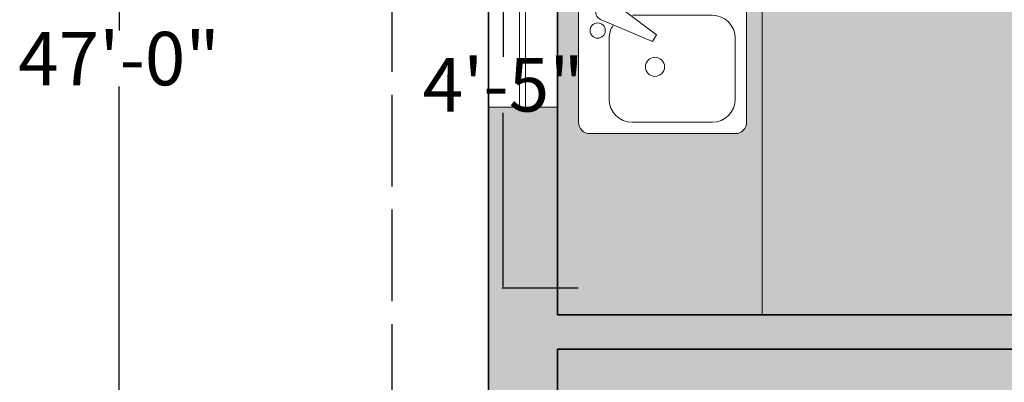
# Model space of a CAD drawing. Units: inches. Extents: x 1316 to 1777, y 813 to 1650.
# Tile 6 of 22: x 1316 to 1445, y 1237 to 1284. Entities that reach past the tile are written whole.
import ezdxf

# ---------------------------------------------------------------- set-up
doc = ezdxf.new("R2010")
doc.units = ezdxf.units.IN
doc.header["$MEASUREMENT"] = 0
doc.linetypes.add('ACAD_ISO02W100', pattern=[15, 12, -3])
for name, color, linetype, lineweight in [('A-ANNO-DIMS', 2, 'Continuous', 18), ('A-FLOR-CASE', 23, 'Continuous', 18), ('A-FLOR-CASE-PATT', 252, 'Continuous', 13), ('A-FLOR-FIXT', 8, 'Continuous', 18), ('A-WALL-PATT', 250, 'Continuous', 13), ('C-PROP', 8, 'ACAD_ISO02W100', 25), ('walls', 250, 'Continuous', 35), ('windows', 141, 'Continuous', 18)]:
    doc.layers.add(name, color=color, linetype=linetype, lineweight=lineweight)
doc.layers.add('A-FLOR-PATT', color=254, linetype='Continuous', lineweight=13, true_color=0xfeeab9)
doc.styles.add('ATT', font='TXT')
doc.styles.get("Standard").update_dxf_attribs({"font": 'arial.ttf'})
doc.dimstyles.get("Standard").update_dxf_attribs({"dimtxt": 7, "dimasz": 0.18, "dimexe": 0.18, "dimexo": 0.0625, "dimgap": 0.09, "dimtad": 0, "dimtih": 1, "dimtoh": 1, "dimzin": 0, "dimdsep": 46, "dimlunit": 3, "dimtxsty": 'Standard', "dimcen": 0.09, "dimadec": 0, "dimazin": 0, "dimtfac": 1, "dimtofl": 0, "dimtmove": 0, "dimatfit": 3, "dimfxl": 1, "dimtolj": 1, "dimtzin": 0, "dimarcsym": 0})

# ---------------------------------------------------------------- blocks, each defined once
blk = doc.blocks.new('15PSNK10')
at = {"color": 0, "linetype": 'ByBlock'}
for p, q in [((20.5, 16.5), (1.5, 16.5)), ((0, 15), (0, -15)), ((7, 15), (17.5, 15)), ((22, -15), (22, 15)), ((4, 4), (4, 12)), ((20.5, 12), (20.5, 4)), ((2.365550999999996, -0.0988979999999984), (2.768423999999995, 0.5988979999999984)), ((10.17820310567643, -3.566986483662404), (4.270020000000002, 0.8709410000000019)), ((17.5, 1), (7, 1)), ((7.038591832997624, -1), (17.5, -1)), ((2.880752999999998, -1.535340000000005), (9.678203105676431, -4.433012483662395)), ((9.678203105676431, -4.433012483662395), (10.17820310567643, -3.566986483662404)), ((4, -12), (4, -4)), ((20.5, -4), (20.5, -12)), ((17.5, -15), (7, -15)), ((1.5, -16.5), (20.5, -16.5))]:
    blk.add_line(p, q, dxfattribs=at)
for centre, radius in [((10, 7.75), 1.25), ((2.5, 3), 1), ((2.5, -3), 1), ((10, -7.75), 1.25)]:
    blk.add_circle(centre, radius, dxfattribs=at)
for centre, radius, start, end in [((1.5, 15), 1.5, 90, 180), ((20.5, 15), 1.5, 0, 90), ((7, 12), 3, 90, 180), ((17.5, 12), 3, 0, 90), ((7, 4), 3, 180, 270), ((17.5, 4), 3, 270, 0), ((3.634449000000003, 0.0988979999999984), 1, 50.537678, 150), ((3.231576000000004, -0.5988979999999984), 1, 150, 249.462322), ((17.5, -4), 3, 0, 90), ((7, -4), 3, 146.6070344853579, 180), ((7, -12), 3, 180, 270), ((17.5, -12), 3, 270, 0), ((1.5, -15), 1.5, 180, 270), ((20.5, -15), 1.5, 270, 0)]:
    blk.add_arc(centre, radius, start, end, dxfattribs=at)
at = {"color": 0, "linetype": 'ByBlock', "style": 'ATT'}
for tag, p, flags in [('ITEM', (0, -26), 3), ('ROOM_NUMBER', (0, -35), 1)]:
    blk.add_attdef(tag, p, '', height=6, dxfattribs=dict(at, flags=flags))
blk = doc.blocks.new('*D23')
at = {"layer": 'A-ANNO-DIMS', "color": 0, "lineweight": -2, "transparency": 16777216}
for p, q in [((1328.466746604303, 1604.172951843256), (1328.865516882555, 1604.172951843256)), ((1328.685516882555, 1603.992951843256), (1328.685516882555, 1282.594977494184)), ((1328.685516882555, 953.868981317008), (1328.685516882555, 1275.26695566608)), ((1328.466746604303, 953.688981317008), (1328.865516882556, 953.688981317008))]:
    blk.add_line(p, q, dxfattribs=at)
at = {"layer": 'A-ANNO-DIMS', "color": 0, "transparency": 16777216}
for points in [[(1328.655516882555, 1603.992951843256), (1328.715516882555, 1603.992951843256), (1328.685516882555, 1604.172951843256)], [(1328.655516882556, 953.868981317008), (1328.715516882555, 953.868981317008), (1328.685516882555, 953.688981317008)]]:
    blk.add_solid(points, dxfattribs=at)
at = {"layer": 'Defpoints', "color": 0, "transparency": 16777216}
for p in [(1328.404246604303, 1604.172951843256), (1328.404246604303, 953.688981317008), (1328.685516882555, 953.688981317008)]:
    blk.add_point(p, dxfattribs=at)
at = {"layer": 'A-ANNO-DIMS', "color": 0, "transparency": 16777216, "insert": (1328.685516882555, 1278.930966580132), "char_height": 7, "width": 24.3281036834925, "attachment_point": 5}
blk.add_mtext('\\A1;47\'-0"', dxfattribs=at)
blk = doc.blocks.new('*D41')
at = {"layer": 'A-ANNO-DIMS', "color": 0, "lineweight": -2, "transparency": 16777216}
for p, q in [((1388.775753781963, 1302.100142632137), (1378.797436635279, 1302.100142632137)), ((1378.977436635279, 1301.920142632137), (1378.977436635279, 1279.143834211486)), ((1378.977436635279, 1249.068153348815), (1378.977436635279, 1271.844461769467)), ((1388.775753781963, 1248.888153348815), (1378.797436635279, 1248.888153348815))]:
    blk.add_line(p, q, dxfattribs=at)
at = {"layer": 'A-ANNO-DIMS', "color": 0, "transparency": 16777216}
for points in [[(1378.947436635279, 1301.920142632137), (1379.007436635279, 1301.920142632137), (1378.977436635279, 1302.100142632137)], [(1378.947436635279, 1249.068153348815), (1379.007436635279, 1249.068153348815), (1378.977436635279, 1248.888153348815)]]:
    blk.add_solid(points, dxfattribs=at)
at = {"layer": 'Defpoints', "color": 0, "transparency": 16777216}
for p in [(1378.977436635279, 1302.100142632137), (1388.838253781963, 1302.100142632137), (1388.838253781963, 1248.888153348815)]:
    blk.add_point(p, dxfattribs=at)
at = {"layer": 'A-ANNO-DIMS', "color": 0, "transparency": 16777216, "insert": (1378.977436635279, 1275.494147990476), "char_height": 7, "attachment_point": 5}
blk.add_mtext('\\A1;4\'-5"', dxfattribs=at)

msp = doc.modelspace()

# ---------------------------------------------------------------- hatches: boundary and pattern name
at = {"layer": 'A-FLOR-CASE-PATT'}
h = msp.add_hatch(color=256, dxfattribs=at)
h.dxf.hatch_style = 1
h.paths.add_polyline_path([(1412.858226839809, 1346.928610372446), (1440.064450217018, 1346.928610372446), (1440.064450217018, 1365.369300926962), (1438.2631613314, 1365.369300926962), (1438.2631613314, 1349.455197936214), (1416.108011424953, 1349.455197936214), (1416.108011424953, 1365.369300926962), (1386.064450217018, 1365.369300926962), (1386.064450217018, 1245.369300926962), (1412.858226839809, 1245.369300926962)])
h.paths.add_polyline_path([(1409.310422891292, 1332.514765372921, -0.4142135623730951), (1410.210422891292, 1331.614765372921), (1410.210422891292, 1311.814765372921, -0.414213562373094), (1409.310422891292, 1310.914765372921), (1389.51042289129, 1310.914765372921, -0.4142135623730959), (1388.61042289129, 1311.814765372921), (1388.61042289129, 1331.614765372921, -0.4142135623730951), (1389.51042289129, 1332.514765372921)], flags=16)
h.paths.add_polyline_path([(1395.986900854525, 1329.42133126595), (1396.276368249055, 1329.76630507332, -0.0171905986958355), (1396.448908786205, 1329.621893017294), (1396.159470211814, 1329.276953556429, -0.2116405901053515), (1397.086205654243, 1327.18561240685, -0.2564460938474173), (1395.778569555149, 1324.8037474367), (1396.003749512095, 1324.413724310425, -0.0171906504505625), (1395.809203446643, 1324.300687980197), (1395.584072921188, 1324.69062548862, -0.550570801787435), (1391.442799396982, 1327.059740487748), (1390.992413104956, 1327.059740487748, -0.0171907290098312), (1390.991493340996, 1327.284740487748), (1391.441732803486, 1327.284740487748, -0.6105283005508269)], flags=0)
h.paths.add_polyline_path([(1395.838098786515, 1327.18561240685, -1), (1392.688098786514, 1327.18561240685, -1)], flags=0)
h.paths.add_polyline_path([(1394.263098786514, 1328.310612406851, -1), (1394.263098786514, 1326.06061240685, -1)], flags=0)
h.paths.add_polyline_path([(1394.263098786514, 1327.973112406851, -1), (1394.263098786514, 1326.39811240685, -1)], flags=0)
h.paths.add_polyline_path([(1407.468247061996, 1327.18561240685, -0.9779444631718501), (1401.824840804736, 1327.059740487748), (1401.37445451271, 1327.059740487748, -0.0171907290098312), (1401.373534748749, 1327.284740487748), (1401.823774211239, 1327.284740487748, -0.9825922263687022)], flags=0)
h.paths.add_polyline_path([(1406.220140194268, 1327.18561240685, -1), (1403.070140194268, 1327.18561240685, -1)], flags=0)
h.paths.add_polyline_path([(1404.645140194268, 1328.310612406851, -1), (1404.645140194268, 1326.06061240685, -1)], flags=0)
h.paths.add_polyline_path([(1404.645140194268, 1327.973112406851, -1), (1404.645140194268, 1326.39811240685, -1)], flags=0)
h.paths.add_polyline_path([(1400.91382896134, 1321.714765372921, -1), (1397.907016821244, 1321.714765372921, -1)], flags=0)
h.paths.add_polyline_path([(1396.101714535222, 1318.885415367262), (1396.391181929752, 1319.230389174631, -0.0171905986957908), (1396.563722466901, 1319.085977118605), (1396.274283892511, 1318.74103765774, -0.2116405901053402), (1397.201019334939, 1316.649696508162, -0.2564460938474829), (1395.893383235845, 1314.267831538011), (1396.11856319279, 1313.877808411735, -0.0171906504505387), (1395.924017127339, 1313.764772081509), (1395.698886601884, 1314.154709589932, -0.5505708017872751), (1391.557613077679, 1316.523824589059), (1391.107226785653, 1316.523824589059, -0.0171907290098486), (1391.106307021692, 1316.748824589059), (1391.556546484182, 1316.748824589059, -0.6105283005510082)], flags=0)
h.paths.add_polyline_path([(1395.952912467211, 1316.649696508162, -1), (1392.802912467211, 1316.649696508162, -1)], flags=0)
h.paths.add_polyline_path([(1407.468247061996, 1316.611253873528, -0.9779444631716472), (1401.824840804736, 1316.485381954425), (1401.37445451271, 1316.485381954425, -0.0171907290098486), (1401.373534748749, 1316.710381954425), (1401.823774211239, 1316.710381954425, -0.9825922263688615)], flags=0)
h.paths.add_polyline_path([(1394.377912467211, 1317.774696508162, -0.9999999703822144), (1394.377912467211, 1315.524696508162, -0.9999999703822144)], flags=0)
h.paths.add_polyline_path([(1394.377912467211, 1317.437196508162, -1), (1394.377912467211, 1315.862196508162, -1)], flags=0)
h.paths.add_polyline_path([(1406.220140194268, 1316.611253873528, -1), (1403.070140194268, 1316.611253873528, -1)], flags=0)
h.paths.add_polyline_path([(1404.645140194268, 1315.486253873528, -0.9999999703822144), (1404.645140194268, 1317.736253873528, -0.9999999703822144)], flags=0)
h.paths.add_polyline_path([(1404.645140194268, 1317.398753873528, -1), (1404.645140194268, 1315.823753873528, -1)], flags=0)
h.paths.add_polyline_path([(1409.338253781963, 1302.100142632137, -0.4142135623730951), (1410.838253781963, 1300.600142632137), (1410.838253781963, 1270.600142632137, -0.4142135623730951), (1409.338253781963, 1269.100142632137), (1390.338253781963, 1269.100142632137, -0.4142135623730951), (1388.838253781963, 1270.600142632137), (1388.838253781963, 1300.600142632137, -0.4142135623730951), (1390.338253781963, 1302.100142632137)], flags=16)
h.paths.add_polyline_path([(1395.838253781963, 1300.600142632137), (1406.338253781963, 1300.600142632137, -0.4142135623730951), (1409.338253781963, 1297.600142632137), (1409.338253781963, 1289.600142632137, -0.4142135623730951), (1406.338253781963, 1286.600142632137), (1395.838253781963, 1286.600142632137, -0.4142135623730951), (1392.838253781963, 1289.600142632137), (1392.838253781963, 1297.600142632137, -0.4142135623730951)], flags=0)
h.paths.add_polyline_path([(1400.088253781963, 1293.350142632137, -1), (1397.588253781963, 1293.350142632137, -1)], flags=0)
h.paths.add_polyline_path([(1392.338253781963, 1288.600142632137, -1), (1390.338253781963, 1288.600142632137, -1)], flags=0)
h.paths.add_polyline_path([(1393.037126479862, 1286.524525876857), (1399.01645688764, 1282.033156148475), (1398.51645688764, 1281.167130148475), (1391.719002681245, 1284.064804380225, -0.4631994748411593), (1391.203386694108, 1285.500520483254), (1391.606259694108, 1286.198316483253, -0.4369421512224802)], flags=0)
h.paths.add_polyline_path([(1392.338253781963, 1282.600142632137, -1), (1390.338253781963, 1282.600142632137, -1)], flags=0)
h.paths.add_polyline_path([(1400.088253781963, 1277.850142632137, -1), (1397.588253781963, 1277.850142632137, -1)], flags=0)
at = {"layer": 'A-FLOR-PATT'}
h = msp.add_hatch(color=256, dxfattribs=at)
h.dxf.hatch_style = 1
h.paths.add_polyline_path([(1567.673142217696, 1281.369300926962), (1651.673142217696, 1281.369300926962), (1651.673142217696, 1365.369300926962), (1597.673142217696, 1365.369300926962), (1597.673142217696, 1429.869300926962), (1570.345136951899, 1429.869300926962), (1570.345136951899, 1471.869300926962), (1510.345136951899, 1471.869300926962), (1510.345136951899, 1429.869300926962), (1444.564450217018, 1429.869300926962), (1444.564450217018, 1322.882360660317), (1444.564450217018, 1300.087519887597), (1510.564450217018, 1300.087519887597), (1510.564450217018, 1295.093869264817), (1510.564450217018, 1240.869300926962), (1386.064450217018, 1240.869300926962), (1386.064450217018, 1171.184826128129), (1400.961298831769, 1171.184826128129), (1400.961298831769, 1106.74181853581), (1386.064450217018, 1106.74181853581), (1386.064450217018, 1072.869300926962), (1510.564450217018, 1072.869300926962), (1510.564450217018, 1040.172951843256), (1541.068383692007, 1040.172951843256, -0.367085007058701), (1572.764174999282, 1069.546549507821), (1572.764174999282, 1069.578525976929), (1574.225256623933, 1069.578525976929), (1574.225256623933, 1040.172951843256), (1616.037285953149, 1040.172951843256), (1616.037285953149, 1086.627161740109), (1616.037285953149, 1103.704513499145), (1613.066060418845, 1105.234780569291), (1616.037285953149, 1106.685539866415), (1616.037285953149, 1123.869300926962), (1567.673142217696, 1123.869300926962)])
h.paths.add_polyline_path([(1508.987494855724, 1198.018101264616), (1511.117481528599, 1198.018101264616), (1511.117481528599, 1200.148087937491), (1532.594847146751, 1200.148087937491), (1532.594847146751, 1198.018101264616), (1534.724833819626, 1198.018101264616), (1534.724833819626, 1176.008238978245), (1530.464860473877, 1176.008238978245), (1530.464860473877, 1176.71823453587), (1513.247468201473, 1176.71823453587), (1513.247468201473, 1176.008238978245), (1508.987494855724, 1176.008238978245)], flags=16)
h.paths.add_polyline_path([(1505.978911344017, 1151.314990471522), (1521.503967005494, 1151.314990471522), (1521.503967005494, 1123.622553675171), (1505.978911344017, 1123.622553675171)], flags=16)
h.paths.add_polyline_path([(1507.734238645614, 1150.100746953806, -1), (1506.932299902515, 1150.100746953806, -1)], flags=0)
h.paths.add_polyline_path([(1512.288074001727, 1138.353334368216), (1512.279600715468, 1138.392440283947), (1512.219350358134, 1138.376242249414)], flags=0)
h.paths.add_polyline_path([(1511.538708600003, 1138.926307509397), (1511.801586230713, 1138.967144364025), (1511.816822451641, 1139.269704188439), (1511.606794574277, 1139.246286533845)], flags=0)
h.paths.add_polyline_path([(1513.744555260512, 1140.234298321423), (1513.680232363733, 1139.885116881769), (1514.013725426534, 1140.045442118172), (1513.85452204526, 1140.307851476896)], flags=0)
h.paths.add_polyline_path([(1513.759454991183, 1139.088508933479), (1514.004707571892, 1139.255238426424), (1513.806733823314, 1139.482778214552), (1513.564128907831, 1139.327271464974)], flags=0)
h.paths.add_polyline_path([(1514.219475210051, 1138.385213274156), (1514.335730050378, 1138.330012877603), (1514.544443105969, 1138.319719602207), (1514.802071501717, 1138.873746829037), (1514.451386945615, 1138.715560522777)], flags=0)
h.paths.add_polyline_path([(1514.576784523415, 1137.439218133731), (1514.572807725035, 1137.400121795131), (1514.699202201671, 1137.400121795131), (1514.696265725507, 1137.401958254237)], flags=0)
h.paths.add_polyline_path([(1512.259630054145, 1136.199252443718), (1512.198645006043, 1136.399020086717), (1512.031969302785, 1136.324884611944), (1512.095408670439, 1136.101205019573), (1512.257489338984, 1136.192116726515)], flags=0)
h.paths.add_polyline_path([(1512.643663084783, 1137.273739653883), (1512.355504649132, 1137.230281342332), (1512.431954114942, 1137.048783229095), (1512.702875297586, 1137.092989450977)], flags=0)
h.paths.add_polyline_path([(1513.048588650928, 1137.592520798729), (1512.979298324136, 1137.799799709794), (1512.842806872769, 1137.757466697763), (1512.887278702865, 1137.556025839099)], flags=0)
h.paths.add_polyline_path([(1513.269281623239, 1138.555876366321), (1513.570749546786, 1137.962332598873), (1513.458764523686, 1136.814048268166), (1513.212081965274, 1137.877990637943), (1513.032322366809, 1138.442602014432)], flags=0)
h.paths.add_polyline_path([(1514.891020715756, 1136.377090047208), (1514.695899864911, 1136.400535518201), (1514.682939550409, 1136.245500587688), (1514.870369662043, 1136.165423867704)], flags=0)
h.paths.add_polyline_path([(1514.142311807212, 1137.292647657223), (1514.047049214511, 1136.74320071616), (1514.270411313405, 1136.750949401328), (1514.327746372416, 1137.265481105849)], flags=0)
h.paths.add_polyline_path([(1515.361925908058, 1138.975942407129), (1515.333738674027, 1138.638448296537), (1515.595602136156, 1138.588081597507), (1515.627104749056, 1138.931608018565)], flags=0)
h.paths.add_polyline_path([(1537.284795120854, 1177.912388692567), (1537.994790678479, 1177.912388692567), (1537.994790678479, 1195.129780964971), (1537.284795120854, 1195.129780964971), (1537.284795120854, 1199.38975431072), (1559.294657407225, 1199.38975431072), (1559.294657407225, 1197.259767637845), (1561.4246440801, 1197.259767637845), (1561.4246440801, 1175.782402019693), (1559.294657407225, 1175.782402019693), (1559.294657407225, 1173.652415346818), (1559.378615070445, 1173.652415346818), (1559.378615070445, 1171.514303738793), (1561.51672667847, 1171.514303738793), (1561.51672667847, 1098.818509065945), (1559.378615070445, 1098.818509065945), (1559.378615070445, 1096.68039745792), (1537.284795120854, 1096.68039745792), (1537.284795120854, 1100.95662067397), (1537.997498990196, 1100.95662067397), (1537.997498990196, 1169.376192130768), (1537.284795120854, 1169.376192130768), (1537.284795120854, 1173.652415346818)], flags=16)
h.paths.add_polyline_path([(1518.623279367581, 1345.565265318288), (1519.133216999197, 1345.479657117201), (1519.133247129367, 1345.484585273925), (1518.623292796693, 1345.567461813277)], flags=16)
h.paths.add_polyline_path([(1518.798043157878, 1374.150014517315), (1519.307980789494, 1374.064406316228), (1519.308010919664, 1374.069334472953), (1518.79805658699, 1374.152211012305)], flags=16)
h.paths.add_polyline_path([(1537.763945546351, 1413.501272593833), (1537.678419015976, 1412.991334462891), (1537.683273643974, 1412.991304782267), (1537.76615767817, 1413.501259069119)], flags=16)
h.paths.add_polyline_path([(1572.904903294898, 1373.821409718101), (1573.926762419731, 1373.974678074354), (1574.026627442758, 1390.308820473798), (1573.007147246318, 1390.474521481455), (1573.006718884663, 1390.474591095266)], flags=16)
h.paths.add_polyline_path([(1572.730139504601, 1345.236660519073), (1573.751998629434, 1345.389928875326), (1573.851863652461, 1361.72407127477), (1572.832383456021, 1361.889772282427), (1572.831955094366, 1361.889841896238)], flags=16)
h.paths.add_polyline_path([(1537.210658487583, 1322.64259197221), (1537.363943428096, 1321.620732745983), (1553.69808582754, 1321.520867722956), (1553.863838585734, 1322.540776390265)], flags=16)
h.paths.add_polyline_path([(1535.907853535946, 1331.328394679552), (1527.214399285865, 1331.381545435045), (1527.663791889487, 1404.885186232545), (1564.415612288236, 1404.660489930734), (1563.966219684615, 1331.156849133235), (1555.272745017813, 1331.210000013553), (1553.946716560728, 1323.050730714162), (1537.134020158137, 1323.153521560007)], flags=16)
h.paths.add_polyline_path([(1536.149948378398, 1336.502989385165), (1536.235164066325, 1337.571577967879), (1536.323287084786, 1338.628101895201), (1536.410786509507, 1339.662781903015), (1536.494625364907, 1340.6698173033), (1536.573878305868, 1341.65983134291), (1536.648126641431, 1342.647834135966), (1536.716972722469, 1343.648937760143), (1536.780017027388, 1344.677948027938), (1536.836830656389, 1345.749875115879), (1536.91349345135, 1347.47536960008), (1536.930181129876, 1348.082213381731), (1536.86671979596, 1346.313806322279), (1536.754065794645, 1344.188314997416), (1536.618602559507, 1342.21851898877), (1536.494625364906, 1340.669817303289), (1536.410786509508, 1339.662781903024), (1536.323287084785, 1338.628101895196), (1536.235164066325, 1337.571577967878), (1536.149948378398, 1336.502989385167), (1536.071202820108, 1335.432319400725), (1536.002480605875, 1334.369653419014), (1535.917201218224, 1332.754159960459), (1535.909282823342, 1332.307756473361), (1535.96435308899, 1333.780079645636), (1536.071202820108, 1335.432319400726)], flags=0)
h.paths.add_polyline_path([(1540.411728678358, 1338.345220732376), (1540.538507986221, 1339.036732867615), (1540.667450686668, 1339.758144792479), (1540.798139602249, 1340.51803480286), (1540.930104638842, 1341.324675241543), (1541.06290820131, 1342.186644529235), (1541.195663950278, 1343.109256879628), (1541.325751198274, 1344.084667215432), (1541.450112594895, 1345.102072455087), (1541.565699126105, 1346.150363189455), (1541.669432399664, 1347.218634373414), (1541.758274858692, 1348.295980712192), (1541.829158319786, 1349.371497098253), (1541.87902418423, 1350.434176273261), (1541.905658245644, 1351.475864398132), (1541.910264078201, 1352.499718972741), (1541.894848813054, 1353.511751165878), (1541.861450207875, 1354.517971959091), (1541.812104772023, 1355.524188157142), (1541.748831093802, 1356.536615043187), (1541.673675267255, 1357.560957271187), (1541.551221046702, 1359.062282646612), (1541.495486505545, 1359.670454934914), (1541.588655256529, 1358.603328035907), (1541.721318618915, 1356.976835527602), (1541.846114060333, 1354.980013725856), (1541.912433480836, 1352.981966815021), (1541.903299375855, 1350.951498912638), (1541.805645357175, 1348.870418133965), (1541.627733180341, 1346.712969607265), (1541.39605931794, 1344.611846225434), (1541.135168242209, 1342.655652549989), (1540.871929016276, 1340.947082961546), (1540.617179283622, 1339.465841984599), (1540.411728678363, 1338.345220732389), (1540.287580984743, 1337.67502977883), (1540.166494164132, 1337.01788791383), (1540.048925605183, 1336.365114503449), (1539.936674201221, 1335.710368832696), (1539.836864251217, 1335.055036635329), (1539.758020939376, 1334.402536924379), (1539.708629238703, 1333.756391050932), (1539.697173498044, 1333.120018277682), (1539.75093556766, 1332.162191347439), (1539.822087714565, 1331.89006440645), (1539.690956844971, 1332.774679737417), (1539.713650637448, 1334.035332547662), (1539.86680860596, 1335.30285325234), (1540.085210789094, 1336.576760560778), (1540.287580984743, 1337.67502977883)], flags=0)
h.paths.add_polyline_path([(1545.598581542273, 1331.583674047033), (1545.601408931398, 1331.616855477121), (1545.614142276281, 1331.689058908809), (1545.736718477884, 1332.197227143153), (1545.766951209007, 1332.331509735297), (1545.840044120643, 1332.681341212682), (1545.924609388668, 1333.114205605127), (1546.015565858785, 1333.613901317454), (1546.107830504227, 1334.163920489319), (1546.196310713542, 1334.747857411176), (1546.27592408412, 1335.349306311069), (1546.341588213349, 1335.951861417042), (1546.388220074462, 1336.539014868746), (1546.411904372759, 1337.098233262493), (1546.413511757999, 1337.631655211558), (1546.395048737181, 1338.145189796344), (1546.358553067975, 1338.644847998394), (1546.30606313221, 1339.136742887642), (1546.239595021565, 1339.626681393686), (1546.161196702551, 1340.120674435653), (1546.072884891005, 1340.624631031533), (1545.887738197254, 1341.63015699768), (1545.717659533451, 1342.62070013092), (1545.546853733249, 1343.94500888803), (1545.431881256549, 1345.533720124316), (1545.403899849759, 1347.401905451854), (1545.417510423816, 1348.013069267128), (1545.410556413592, 1346.957478372932), (1545.425070640934, 1345.988432507364), (1545.462877367243, 1345.105410056077), (1545.521092971858, 1344.300975918152), (1545.595702123642, 1343.566272620922), (1545.68263719895, 1342.892238827028), (1545.777872657803, 1342.270017126221), (1545.877351709551, 1341.690648207114), (1545.977037981224, 1341.145172633476), (1546.133225269608, 1340.296924301995), (1546.32712189736, 1339.07516870602), (1546.43378476773, 1337.614859053002), (1546.377188266119, 1336.278538916938), (1546.246417261819, 1335.078542247844), (1546.032296532176, 1333.665423983985), (1545.840044120643, 1332.681341212682), (1545.766951209007, 1332.331509735297)], flags=0)
h.paths.add_polyline_path([(1551.802739251137, 1337.655775652498), (1551.96257269545, 1338.249893918501), (1552.102195298518, 1338.801154932478), (1552.224958021371, 1339.338328209144), (1552.330696453755, 1339.864579612065), (1552.418402861907, 1340.377056720641), (1552.487067639598, 1340.872600849098), (1552.535672844225, 1341.34835963925), (1552.563199284875, 1341.801276556129), (1552.568639227787, 1342.228499179132), (1552.550972857889, 1342.626868884903), (1552.509678498417, 1342.994551203202), (1552.446288501197, 1343.33337442512), (1552.362792521005, 1343.646491244529), (1552.261208966661, 1343.936747902882), (1552.143557495304, 1344.207194818415), (1552.011836098078, 1344.460678357413), (1551.868075265113, 1344.700350964085), (1551.746105860759, 1344.881722683215), (1550.887297650741, 1346.05192221882), (1550.42788872704, 1347.125680184261), (1550.183287427721, 1348.353333686171), (1550.047936052465, 1349.632359022536), (1549.978096005541, 1351.223542107026), (1549.974102148838, 1353.140827975589), (1549.989226669163, 1353.748427546368), (1549.975058438592, 1352.681752708607), (1549.977087298692, 1351.70778065901), (1549.995607655661, 1350.824569845699), (1550.030618304039, 1350.026913573531), (1550.082058657804, 1349.309911787039), (1550.149928759809, 1348.668561967865), (1550.234168024029, 1348.097964060535), (1550.334775869163, 1347.593013458303), (1550.451691709185, 1347.148810105696), (1550.584412233058, 1346.759844100773), (1550.73038050297, 1346.418678345312), (1550.88655602074, 1346.117266144286), (1551.049909745336, 1345.847764917032), (1551.217401178577, 1345.602127968521), (1551.385990446439, 1345.372410692116), (1551.55262809021, 1345.150770631988), (1552.000038284146, 1344.537104232464), (1552.453505275841, 1343.494713960715), (1552.591463897673, 1342.266339273388), (1552.508711326437, 1340.904737898757), (1552.245597777252, 1339.367339734202), (1551.924893638995, 1338.101128644033), (1551.618511514029, 1336.984114361546), (1551.405674157756, 1336.200020283199), (1551.009764092749, 1334.698598399404), (1550.877399289293, 1334.154667887629), (1551.263664389663, 1335.676855458292), (1551.618511514027, 1336.984114361536)], flags=0)
h.paths.add_polyline_path([(1558.642358998526, 1348.348341932098), (1558.795153425402, 1348.811416841303), (1558.918173552255, 1349.215358215379), (1559.008026171039, 1349.574581801048), (1559.061298904339, 1349.903707646641), (1559.075825921932, 1350.214183320864), (1559.054343192669, 1350.505992096326), (1559.00083323259, 1350.775944766007), (1558.919250427844, 1351.021260663692), (1558.81356708563, 1351.238750644777), (1558.687756761463, 1351.425429741436), (1558.545793010855, 1351.578312985846), (1558.391628971643, 1351.694415535011), (1558.228764001313, 1351.771674150153), (1558.05869086465, 1351.812121548804), (1557.882428128411, 1351.81871217754), (1557.700994359352, 1351.79440048294), (1557.515397915392, 1351.742140973996), (1557.326668820441, 1351.665092211649), (1557.135793766425, 1351.566004652943), (1556.943823194933, 1351.44803673399), (1556.751584825563, 1351.314654529213), (1556.741969848742, 1351.307485185875), (1556.174649390243, 1350.878470713214), (1555.982386678774, 1350.741107061228), (1555.790208852573, 1350.61762743028), (1555.103431920574, 1350.247624890473), (1554.019478994433, 1350.696346369238), (1553.658410413117, 1351.73359972735), (1553.592207666961, 1352.861368347784), (1553.704659497418, 1354.248209262139), (1553.753119918252, 1354.656598557367), (1553.684819216316, 1354.00352392911), (1553.637913725648, 1353.425049987856), (1553.614699631385, 1352.917691559993), (1553.614827379228, 1352.476039895736), (1553.637249468889, 1352.094077959223), (1553.680938817757, 1351.765788589762), (1553.744858758541, 1351.485256777466), (1553.82798220863, 1351.246465361642), (1553.929261667735, 1351.043397306428), (1554.04767130156, 1350.870239627912), (1554.182026927633, 1350.721997047951), (1554.330490954936, 1350.598680801359), (1554.491077653114, 1350.501119766308), (1554.661792955443, 1350.430449148551), (1554.840661964566, 1350.387599852234), (1555.02568040492, 1350.373707145527), (1555.214873379145, 1350.389701932573), (1555.406255781046, 1350.436515179933), (1555.598153361026, 1350.514157123772), (1555.790208852573, 1350.61762743028), (1555.982386678773, 1350.741107061227), (1556.174649390244, 1350.878470713214), (1556.366961410069, 1351.02389934801), (1556.559285288865, 1351.171267662216), (1556.751584825563, 1351.314654529213), (1556.943823194933, 1351.44803673399), (1557.135793766425, 1351.566004652943), (1557.326668820441, 1351.665092211648), (1558.042515074605, 1351.95733685961), (1558.893728230531, 1351.316279335487), (1559.136865914879, 1350.089672795452), (1558.886015641058, 1349.086793457618), (1558.642358998525, 1348.348341932093), (1558.463193064356, 1347.811615590227), (1558.261048830942, 1347.186822068983), (1558.03933929985, 1346.459443408408), (1557.677450203418, 1345.174834336041), (1557.548968991007, 1344.635807724703), (1557.908545731516, 1346.030339390738), (1558.328508124364, 1347.408140702653)], flags=0)
h.paths.add_polyline_path([(1562.145123345359, 1353.919129120074), (1562.250304117219, 1354.679787637482), (1562.34093833006, 1355.343853771733), (1562.416101040585, 1355.923686334763), (1562.475035862508, 1356.430826370303), (1562.517611688201, 1356.872216949942), (1562.54387555173, 1357.25388122627), (1562.553854069482, 1357.581842476714), (1562.547593651368, 1357.862021765479), (1562.525120913776, 1358.10044236999), (1562.486482890773, 1358.30312744284), (1562.431704950433, 1358.475896084676), (1562.361155192264, 1358.623850655281), (1562.276503898586, 1358.748001864806), (1562.179752001843, 1358.848337479786), (1562.072869183806, 1358.924743365611), (1561.957877418753, 1358.977309252376), (1561.836746388454, 1359.005921005473), (1561.71148785835, 1359.010668417409), (1561.584092552045, 1358.991539317136), (1561.456045120288, 1358.949239273116), (1561.341584300566, 1358.895014406292), (1560.779829007024, 1358.553784684453), (1560.630616275888, 1358.472819004295), (1560.474487483611, 1358.402819474164), (1560.311154867376, 1358.348484094885), (1559.637466910391, 1358.206630908504), (1558.973121038646, 1358.903907683205), (1558.815552073528, 1360.002456271339), (1558.803942930122, 1361.236291863163), (1558.829841213422, 1361.673699707903), (1558.80694301689, 1360.917438550413), (1558.812784665874, 1360.296580130481), (1558.845278068372, 1359.795210830316), (1558.902335132382, 1359.397417032129), (1558.981856932905, 1359.087183092155), (1559.081756002095, 1358.848697480995), (1559.199942999639, 1358.66584240408), (1559.334180223548, 1358.524951186848), (1559.481597784608, 1358.420834672959), (1559.639186392453, 1358.350550586885), (1559.803946965561, 1358.311156590683), (1559.97287021357, 1358.299710408824), (1560.142945597805, 1358.313065589002), (1560.311154867377, 1358.348484094885), (1560.474487483611, 1358.402819474164), (1560.630616275888, 1358.472819004295), (1560.779829007024, 1358.553784684454), (1560.923096183733, 1358.640810155187), (1561.061387688574, 1358.728886968651), (1561.195663195268, 1358.813006739421), (1561.382100208996, 1358.919625179564), (1561.341584300566, 1358.895014406292), (1561.972476451099, 1359.193894345525), (1562.53631106285, 1358.366963698877), (1562.559911530188, 1357.31074636116), (1562.455247211757, 1356.225674176933), (1562.323097858171, 1355.206225864646), (1562.145123345359, 1353.91912912008), (1562.026320333625, 1353.049417319218), (1561.815039989057, 1351.456922136686), (1561.751502783429, 1350.932786338753), (1561.948339842468, 1352.478551712307)], flags=0)
h.paths.add_polyline_path([(1572.764174999282, 1069.546549507821, 0.3670850070587006), (1541.068383692007, 1040.172951843256), (1572.764174999282, 1040.172951843256)], flags=17)
h.paths.add_polyline_path([(1572.764174999282, 1040.172951843256), (1541.068383692007, 1040.172951843256, 0.0299535364659094), (1540.829105203347, 1036.182374556343), (1540.829105203347, 1031.172951843255), (1574.225256623933, 1031.172951843255), (1574.225256623933, 1036.182374556343), (1572.764174999282, 1036.182374556343)])
h = msp.add_hatch(color=256, dxfattribs=at)
h.dxf.hatch_style = 1
h.paths.add_polyline_path([(1506.064450217018, 1295.093869264817), (1444.564450217018, 1295.093869264817), (1444.564450217018, 1322.882360660317), (1440.064450217018, 1322.882360660317), (1440.064450217018, 1346.928610372446), (1412.858226839809, 1346.928610372446), (1412.858226839809, 1245.369300926962), (1506.064450217018, 1245.369300926962)])
h.paths.add_polyline_path([(1484.664907055627, 1269.305233675322), (1504.590417462121, 1269.305233675322), (1504.590417462121, 1245.841035562835), (1484.664907055627, 1245.841035562835)], flags=16)
h.paths.add_polyline_path([(1510.564450217018, 1300.087519887597), (1444.564450217018, 1300.087519887597), (1444.564450217018, 1295.093869264817), (1506.064450217018, 1295.093869264817), (1510.564450217018, 1295.093869264817)])
at = {"layer": 'A-WALL-PATT'}
h = msp.add_hatch(color=256, dxfattribs=at)
h.dxf.hatch_style = 1
h.paths.add_polyline_path([(1713.173142217696, 1281.369300926962), (1656.173142217696, 1281.369300926962), (1656.173142217696, 1298.257717658217), (1651.673142217696, 1298.257717658217), (1651.673142217696, 1281.369300926962), (1567.673142217696, 1281.369300926962), (1567.673142217696, 1266.995117174766), (1572.173142217695, 1266.995117174766), (1572.173142217695, 1276.869300926963), (1704.173142217696, 1276.869300926962), (1704.173142217696, 1132.869300926962), (1608.640148269009, 1132.869300926962), (1608.640148269009, 1123.869300926962), (1704.173142217696, 1123.869300926962), (1704.173142217696, 1040.172951843256), (1652.868762127258, 1040.172951843256), (1652.868762127258, 1031.172951843254), (1713.173142217696, 1031.172951843253), (1713.173142217696, 1040.172951843256)])
h.paths.add_polyline_path([(1572.173142217696, 1237.954794134253), (1567.673142217696, 1237.954794134253), (1567.673142217696, 1123.869300926962), (1583.145592691861, 1123.869300926962), (1583.145592691861, 1132.869300926963), (1572.173142217696, 1132.869300926963)], flags=17)
h.paths.add_polyline_path([(1510.345136951899, 1566.369300926962), (1524.170902149835, 1566.369300926962), (1524.170902149835, 1571.984613741441), (1524.170902149835, 1575.369300926961), (1445.954793584458, 1575.369300926961), (1445.954793584458, 1566.369300926962), (1505.845136951899, 1566.369300926962), (1505.845136951899, 1469.591483064839), (1510.345136951899, 1469.591483064839), (1510.345136951899, 1471.869300926962), (1529.081211183796, 1471.869300926962), (1529.081211183796, 1476.369300926962), (1510.345136951899, 1476.369300926962)])
h.paths.add_polyline_path([(1609.722471703215, 1575.369300926961), (1545.118796217357, 1575.369300926961), (1545.118796217357, 1566.369300926962), (1570.345136951899, 1566.369300926962), (1570.345136951899, 1476.369300926962), (1562.477362604382, 1476.369300926962), (1562.477362604382, 1471.869300926962), (1570.345136951899, 1471.869300926962), (1570.345136951899, 1469.591483064839), (1574.845136951899, 1469.591483064839), (1574.845136951899, 1566.369300926962), (1609.722471703215, 1566.369300926962)])
h.paths.add_polyline_path([(1713.173142217696, 1575.369300926961), (1655.232651300773, 1575.369300926961), (1655.232651300773, 1566.369300926962), (1704.173142217696, 1566.369300926962), (1704.173142217696, 1434.369300926962), (1574.845136951899, 1434.369300926962), (1574.845136951899, 1440.551160024325), (1574.701185407976, 1440.551160024325), (1570.345136951899, 1440.551160024325), (1570.345136951899, 1429.869300926962), (1597.673142217696, 1429.869300926962), (1597.673142217696, 1408.281186528541), (1602.173142217695, 1408.281186528541), (1602.173142217695, 1429.869300926962), (1704.173142217696, 1429.869300926962), (1704.173142217696, 1410.703982852585), (1707.374745037781, 1410.703982852585), (1713.173142217696, 1410.703982852585)])
h.paths.add_polyline_path([(1713.173142217696, 1383.675544097327), (1704.173142217696, 1383.675544097327), (1704.173142217696, 1369.869300926962), (1602.173142217696, 1369.869300926962), (1602.173142217695, 1379.240863488028), (1597.673142217696, 1379.240863488028), (1597.673142217696, 1365.369300926962), (1713.173142217696, 1365.369300926962)])
h.paths.add_polyline_path([(1444.564450217018, 1429.869300926962), (1510.345136951899, 1429.869300926962), (1510.345136951899, 1440.551160024325), (1505.845136951899, 1440.551160024325), (1505.845136951899, 1434.369300926962), (1386.064450217018, 1434.369300926961), (1386.064450217018, 1566.369300926962), (1400.4446139869, 1566.369300926962), (1400.4446139869, 1575.369300926961), (1377.064450217018, 1575.369300926961), (1377.064450217018, 1412.813262305812), (1380.508552477466, 1412.813262305812), (1386.064450217018, 1412.813262305812), (1386.064450217018, 1429.869300926962), (1440.064450217018, 1429.869300926962), (1440.064450217018, 1401.229090636953), (1444.564450217018, 1401.229090636953)])
h.paths.add_polyline_path([(1444.564450217018, 1372.18876759644), (1440.064450217018, 1372.18876759644), (1440.064450217018, 1369.869300926962), (1386.064450217018, 1369.869300926962), (1386.064450217018, 1378.757622609401), (1377.064450217018, 1378.757622609401), (1377.064450217018, 1349.201183977028), (1381.117947355797, 1349.201183977028), (1386.064450217018, 1349.201183977028), (1386.064450217018, 1365.369300926962), (1440.064450217018, 1365.369300926962), (1440.064450217018, 1322.882360660317), (1444.564450217018, 1322.882360660317)])
h.paths.add_polyline_path([(1510.564450217018, 1295.093869264817), (1506.064450217018, 1295.093869264817), (1506.064450217018, 1245.369300926962), (1386.064450217018, 1245.369300926962), (1386.064450217018, 1272.58216425724), (1377.064450217018, 1272.58216425724), (1377.064450217018, 1212.904590025772), (1380.100240558029, 1212.904590025772), (1386.064450217018, 1212.904590025772), (1386.064450217018, 1240.869300926962), (1510.564450217018, 1240.869300926962)])
h.paths.add_polyline_path([(1386.064450217018, 1163.761289951094), (1377.064450217018, 1163.761289951094), (1377.064450217018, 1063.869300926961), (1419.36334498438, 1063.869300926961), (1419.36334498438, 1072.869300926962), (1386.064450217018, 1072.869300926962)])
h.paths.add_polyline_path([(1510.564450217018, 1072.869300926962), (1469.381492401113, 1072.869300926962), (1469.381492401113, 1063.869300926961), (1501.564450217018, 1063.869300926962), (1501.564450217018, 1033.022564166395), (1501.564450217018, 1031.172951843256), (1540.829105203347, 1031.172951843255), (1540.829105203347, 1036.182374556343, -0.0299535364659092), (1541.068383692007, 1040.172951843256), (1510.564450217018, 1040.172951843256)])
h.paths.add_polyline_path([(1607.368796217357, 1040.172951843256), (1574.225256623933, 1040.172951843256), (1574.225256623933, 1036.182374556343), (1574.225256623933, 1031.172951843255), (1607.368796217357, 1031.172951843254)], flags=17)
h.paths.add_polyline_path([(1637.054389108292, 1040.172951843256), (1624.70577568894, 1040.172951843256), (1624.70577568894, 1031.172951843254), (1637.054389108293, 1031.172951843254)], flags=17)

# ---------------------------------------------------------------- linework, layer by layer
at = {"layer": 'A-FLOR-CASE'}
msp.add_line((1412.858226839809, 1346.928610372446), (1412.858226839809, 1245.369300926962), dxfattribs=at)
at = {"layer": 'C-PROP'}
msp.add_line((1364.398563382318, 1604.172951843256), (1364.398563382318, 953.6889813170072), dxfattribs=at)
at = {"layer": 'walls'}
for p, q in [((1377.064450217018, 1575.369300926961), (1377.064450217018, 953.6889813170072)), ((1386.064450217018, 1365.369300926962), (1386.064450217018, 1245.369300926962)), ((1386.064450217018, 1245.369300926962), (1506.064450217018, 1245.369300926962)), ((1386.064450217018, 1240.869300926962), (1510.564450217018, 1240.869300926962)), ((1386.064450217018, 1240.869300926961), (1386.064450217018, 1072.869300926962))]:
    msp.add_line(p, q, dxfattribs=at)
at = {"layer": 'windows'}
for p, q in [((1381.117947355797, 1349.201183977028), (1381.117947355797, 1272.58216425724)), ((1381.904112948374, 1272.58216425724), (1381.904112948374, 1349.201183977028)), ((1386.064450217018, 1349.201183977028), (1386.064450217018, 1272.58216425724)), ((1377.064450217018, 1272.58216425724), (1377.064450217018, 1344.130177497399)), ((1386.064450217018, 1272.58216425724), (1377.064450217018, 1272.58216425724)), ((1381.117947355797, 1272.58216425724), (1381.904112948374, 1272.58216425724))]:
    msp.add_line(p, q, dxfattribs=at)

# ---------------------------------------------------------------- block references
at = {"layer": 'A-FLOR-FIXT'}
msp.add_blockref('15PSNK10', (1388.838253781963, 1285.600142632137), dxfattribs=at)

# ---------------------------------------------------------------- dimensions: what is measured, and where the dimension line sits
at = {"layer": 'A-ANNO-DIMS'}
dim = msp.add_linear_dim(base=(1328.685516882555, 953.688981317008), p1=(1328.404246604303, 1604.172951843256), p2=(1328.404246604303, 953.6889813170077), angle=90, text='47\'-0"', dimstyle='Standard', override={"dimclrd": 0, "dimclre": 0, "dimclrt": 0}, dxfattribs=at)
dim.commit()
dim.dimension.update_dxf_attribs({"geometry": '*D23', "text_midpoint": (1328.685516882555, 1278.930966580132)})
dim = msp.add_linear_dim(base=(1378.977436635279, 1302.100142632137), p1=(1388.838253781963, 1248.888153348814), p2=(1388.838253781963, 1302.100142632137), angle=90, dimstyle='Standard', override={"dimdec": 1, "dimlfac": 1, "dimrnd": 0, "dimzin": 1, "dimdsep": 46, "dimlunit": 4, "dimfrac": 2}, dxfattribs=at)
dim.commit()
dim.dimension.update_dxf_attribs({"geometry": '*D41', "text_midpoint": (1378.977436635279, 1275.494147990476)})

doc.saveas('drawing.dxf')
